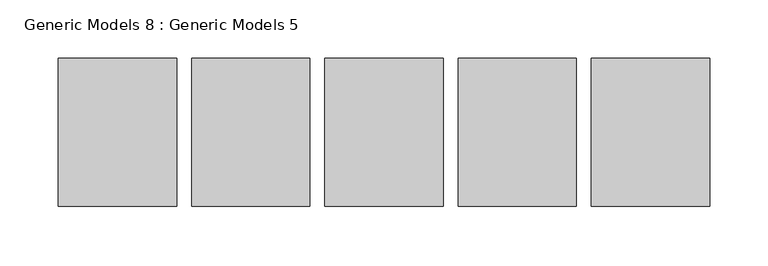
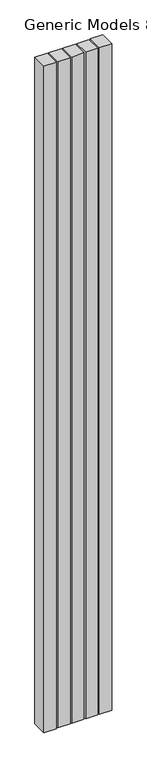
"""IFC4 building model written with IfcOpenShell, lengths in millimetres: proxy geometry, Generic Models 8 : Generic Models 5."""

from ifc_helpers import new_model, si_unit, frame, origin, place, context, project, spatial, polyline, outline, extrude, source, transform, mapped, element, save


def generic_models_8_generic_models_5_f34dc4a4(model_context):
    return source(origin(), model_context, "Body", "SweptSolid", [
        extrude(outline(polyline([(-3148.321199, -5879.7642512), (-3249.921199, -5879.7642512), (-3249.921199, -5752.7642512), (-3148.321199, -5752.7642512), (-3148.321199, -5879.7642512)])), frame((0.0, 0.0, 304.8), z_axis=(0.0, 0.0, 1.0), x_axis=(1.0, 0.0, 0.0)), (0.0, 0.0, 1.0), 5798.7761011),
        extrude(outline(polyline([(-3034.021199, -5879.7642512), (-3135.621199, -5879.7642512), (-3135.621199, -5752.7642512), (-3034.021199, -5752.7642512), (-3034.021199, -5879.7642512)])), frame((0.0, 0.0, 304.8), z_axis=(0.0, 0.0, 1.0), x_axis=(1.0, 0.0, 0.0)), (0.0, 0.0, 1.0), 5798.7761011),
        extrude(outline(polyline([(-2919.721199, -5879.7642512), (-3021.321199, -5879.7642512), (-3021.321199, -5752.7642512), (-2919.721199, -5752.7642512), (-2919.721199, -5879.7642512)])), frame((0.0, 0.0, 304.8), z_axis=(0.0, 0.0, 1.0), x_axis=(1.0, 0.0, 0.0)), (0.0, 0.0, 1.0), 5798.7761011),
        extrude(outline(polyline([(-2805.421199, -5879.7642512), (-2907.021199, -5879.7642512), (-2907.021199, -5752.7642512), (-2805.421199, -5752.7642512), (-2805.421199, -5879.7642512)])), frame((0.0, 0.0, 304.8), z_axis=(0.0, 0.0, 1.0), x_axis=(1.0, 0.0, 0.0)), (0.0, 0.0, 1.0), 5798.7761011),
        extrude(outline(polyline([(-2691.121199, -5879.7642512), (-2792.721199, -5879.7642512), (-2792.721199, -5752.7642512), (-2691.121199, -5752.7642512), (-2691.121199, -5879.7642512)])), frame((0.0, 0.0, 304.8), z_axis=(0.0, 0.0, 1.0), x_axis=(1.0, 0.0, 0.0)), (0.0, 0.0, 1.0), 5798.7761011),
    ])


if __name__ == "__main__":
    model = new_model("IFC4")
    model_context = context("Model", 3, world=origin())
    ifc_project = project(units=[si_unit("LENGTHUNIT", "METRE", prefix="MILLI")], contexts=[model_context])
    site = spatial("IfcSite", under=ifc_project)
    building = spatial("IfcBuilding", under=site)
    placement = place(None, origin())
    generic_models_8_generic_models_5_shape = generic_models_8_generic_models_5_f34dc4a4(model_context)
    element("IfcBuildingElementProxy", 1, Name="Generic Models 8 : Generic Models 5", ObjectType="Generic Models 8 : Generic Models 5", at=placement, inside=building, context=model_context, shape_type="MappedRepresentation", body=[
        mapped(generic_models_8_generic_models_5_shape, transform((0.0, 0.0, 0.0), x_axis=(1.0, 0.0, 0.0), y_axis=(0.0, 1.0, 0.0), z_axis=(0.0, 0.0, 1.0))),
    ])
    save(model, "model.ifc")
